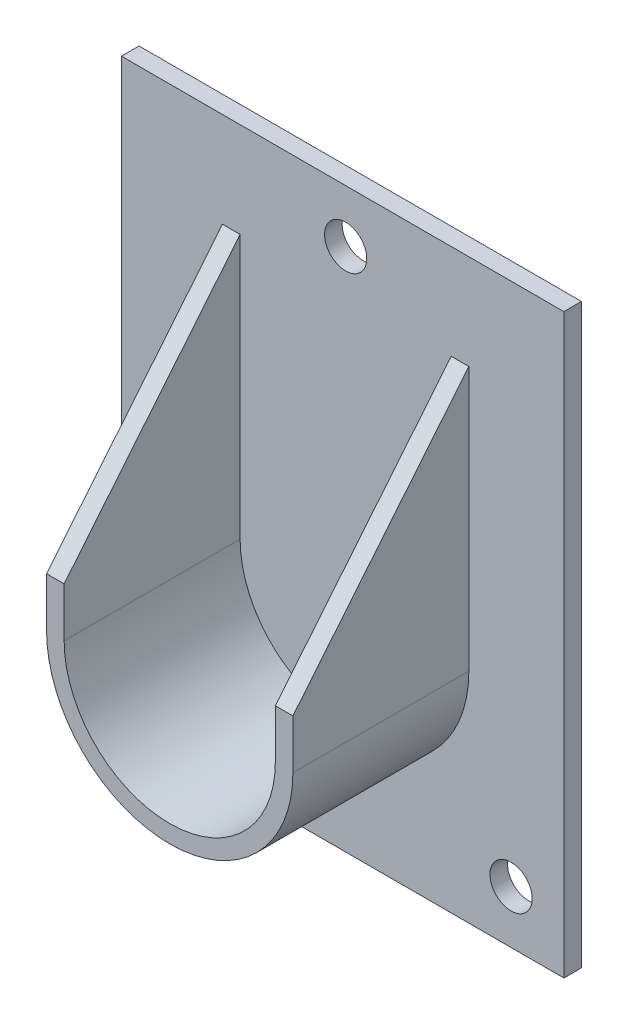
ISO-10303-21;
HEADER;
FILE_DESCRIPTION(('STEP AP214'),'2;1');
FILE_NAME('part.step','',(''),(''),'','','');
FILE_SCHEMA(('AUTOMOTIVE_DESIGN { 1 0 10303 214 1 1 1 1 }'));
ENDSEC;
DATA;
#1=APPLICATION_CONTEXT('core data for automotive mechanical design processes');
#2=APPLICATION_PROTOCOL_DEFINITION('international standard','automotive_design',2000,#1);
#3=PRODUCT_CONTEXT('',#1,'mechanical');
#4=PRODUCT('Part','Part','',(#3));
#5=PRODUCT_RELATED_PRODUCT_CATEGORY('part','',(#4));
#6=PRODUCT_DEFINITION_FORMATION('','',#4);
#7=PRODUCT_DEFINITION_CONTEXT('part definition',#1,'design');
#8=PRODUCT_DEFINITION('design','',#6,#7);
#9=PRODUCT_DEFINITION_SHAPE('','',#8);
#10=(LENGTH_UNIT() NAMED_UNIT(*) SI_UNIT(.MILLI.,.METRE.));
#11=(NAMED_UNIT(*) PLANE_ANGLE_UNIT() SI_UNIT($,.RADIAN.));
#12=(NAMED_UNIT(*) SI_UNIT($,.STERADIAN.) SOLID_ANGLE_UNIT());
#13=UNCERTAINTY_MEASURE_WITH_UNIT(LENGTH_MEASURE(1.E-05),#10,'distance_accuracy_value','');
#14=(GEOMETRIC_REPRESENTATION_CONTEXT(3) GLOBAL_UNCERTAINTY_ASSIGNED_CONTEXT((#13)) GLOBAL_UNIT_ASSIGNED_CONTEXT((#10,
#11,#12)) REPRESENTATION_CONTEXT('',''));
#15=CARTESIAN_POINT('',(0.,0.,0.));
#16=DIRECTION('',(0.,0.,1.));
#17=DIRECTION('',(1.,0.,0.));
#18=AXIS2_PLACEMENT_3D('',#15,#16,#17);
#19=CARTESIAN_POINT('',(0.,0.,55.));
#20=DIRECTION('',(0.,0.,-1.));
#21=DIRECTION('',(-1.,0.,0.));
#22=AXIS2_PLACEMENT_3D('',#19,#20,#21);
#23=CYLINDRICAL_SURFACE('',#22,30.);
#24=DIRECTION('',(0.,0.,-1.));
#25=VECTOR('',#24,1.);
#26=CARTESIAN_POINT('',(30.,0.,55.));
#27=LINE('',#26,#25);
#28=CARTESIAN_POINT('',(30.,0.,55.));
#29=VERTEX_POINT('',#28);
#30=CARTESIAN_POINT('',(30.,0.,5.));
#31=VERTEX_POINT('',#30);
#32=EDGE_CURVE('E156',#29,#31,#27,.T.);
#33=ORIENTED_EDGE('',*,*,#32,.T.);
#34=CARTESIAN_POINT('',(0.,0.,5.));
#35=DIRECTION('',(0.,0.,-1.));
#36=DIRECTION('',(-1.,0.,0.));
#37=AXIS2_PLACEMENT_3D('',#34,#35,#36);
#38=CIRCLE('',#37,30.);
#39=CARTESIAN_POINT('',(-30.,0.,5.));
#40=VERTEX_POINT('',#39);
#41=EDGE_CURVE('E52',#31,#40,#38,.T.);
#42=ORIENTED_EDGE('',*,*,#41,.T.);
#43=DIRECTION('',(0.,0.,-1.));
#44=VECTOR('',#43,1.);
#45=CARTESIAN_POINT('',(-30.,0.,55.));
#46=LINE('',#45,#44);
#47=CARTESIAN_POINT('',(-30.,0.,55.));
#48=VERTEX_POINT('',#47);
#49=EDGE_CURVE('E46',#48,#40,#46,.T.);
#50=ORIENTED_EDGE('',*,*,#49,.F.);
#51=CARTESIAN_POINT('',(0.,0.,55.));
#52=DIRECTION('',(0.,0.,1.));
#53=DIRECTION('',(1.,0.,0.));
#54=AXIS2_PLACEMENT_3D('',#51,#52,#53);
#55=CIRCLE('',#54,30.);
#56=EDGE_CURVE('E170',#48,#29,#55,.T.);
#57=ORIENTED_EDGE('',*,*,#56,.T.);
#58=EDGE_LOOP('',(#33,#42,#50,#57));
#59=FACE_BOUND('',#58,.T.);
#60=ADVANCED_FACE('F39',(#59),#23,.F.);
#61=CARTESIAN_POINT('',(-30.,0.,55.));
#62=DIRECTION('',(-1.,0.,0.));
#63=DIRECTION('',(0.,0.,1.));
#64=AXIS2_PLACEMENT_3D('',#61,#62,#63);
#65=PLANE('',#64);
#66=DIRECTION('',(0.,-1.,0.));
#67=VECTOR('',#66,1.);
#68=CARTESIAN_POINT('',(-30.,0.,5.));
#69=LINE('',#68,#67);
#70=CARTESIAN_POINT('',(-30.,75.,5.));
#71=VERTEX_POINT('',#70);
#72=EDGE_CURVE('E176',#71,#40,#69,.T.);
#73=ORIENTED_EDGE('',*,*,#72,.F.);
#74=DIRECTION('',(0.,-0.773392104960213,0.63392795488542));
#75=VECTOR('',#74,1.);
#76=CARTESIAN_POINT('',(-30.,5.62610512779296,61.8638482559074));
#77=LINE('',#76,#75);
#78=CARTESIAN_POINT('',(-30.,14.,55.));
#79=VERTEX_POINT('',#78);
#80=EDGE_CURVE('E139',#71,#79,#77,.T.);
#81=ORIENTED_EDGE('',*,*,#80,.T.);
#82=DIRECTION('',(0.,1.,0.));
#83=VECTOR('',#82,1.);
#84=CARTESIAN_POINT('',(-30.,0.,55.));
#85=LINE('',#84,#83);
#86=EDGE_CURVE('E148',#48,#79,#85,.T.);
#87=ORIENTED_EDGE('',*,*,#86,.F.);
#88=ORIENTED_EDGE('',*,*,#49,.T.);
#89=EDGE_LOOP('',(#73,#81,#87,#88));
#90=FACE_BOUND('',#89,.T.);
#91=ADVANCED_FACE('F260',(#90),#65,.F.);
#92=CARTESIAN_POINT('',(-35.,0.,55.));
#93=DIRECTION('',(-1.,0.,0.));
#94=DIRECTION('',(0.,0.,1.));
#95=AXIS2_PLACEMENT_3D('',#92,#93,#94);
#96=PLANE('',#95);
#97=DIRECTION('',(0.,-0.773392104960213,0.63392795488542));
#98=VECTOR('',#97,1.);
#99=CARTESIAN_POINT('',(-35.,5.62610512779296,61.8638482559074));
#100=LINE('',#99,#98);
#101=CARTESIAN_POINT('',(-35.,75.,5.));
#102=VERTEX_POINT('',#101);
#103=CARTESIAN_POINT('',(-35.,14.,55.));
#104=VERTEX_POINT('',#103);
#105=EDGE_CURVE('E127',#102,#104,#100,.T.);
#106=ORIENTED_EDGE('',*,*,#105,.F.);
#107=DIRECTION('',(0.,-1.,0.));
#108=VECTOR('',#107,1.);
#109=CARTESIAN_POINT('',(-35.,0.,5.));
#110=LINE('',#109,#108);
#111=CARTESIAN_POINT('',(-35.,0.,5.));
#112=VERTEX_POINT('',#111);
#113=EDGE_CURVE('E181',#102,#112,#110,.T.);
#114=ORIENTED_EDGE('',*,*,#113,.T.);
#115=DIRECTION('',(0.,0.,-1.));
#116=VECTOR('',#115,1.);
#117=CARTESIAN_POINT('',(-35.,0.,55.));
#118=LINE('',#117,#116);
#119=CARTESIAN_POINT('',(-35.,0.,55.));
#120=VERTEX_POINT('',#119);
#121=EDGE_CURVE('E155',#120,#112,#118,.T.);
#122=ORIENTED_EDGE('',*,*,#121,.F.);
#123=DIRECTION('',(0.,1.,0.));
#124=VECTOR('',#123,1.);
#125=CARTESIAN_POINT('',(-35.,0.,55.));
#126=LINE('',#125,#124);
#127=EDGE_CURVE('E145',#120,#104,#126,.T.);
#128=ORIENTED_EDGE('',*,*,#127,.T.);
#129=EDGE_LOOP('',(#106,#114,#122,#128));
#130=FACE_BOUND('',#129,.T.);
#131=ADVANCED_FACE('F147',(#130),#96,.T.);
#132=CARTESIAN_POINT('',(0.,0.,55.));
#133=DIRECTION('',(0.,0.,-1.));
#134=DIRECTION('',(-1.,0.,0.));
#135=AXIS2_PLACEMENT_3D('',#132,#133,#134);
#136=CYLINDRICAL_SURFACE('',#135,35.);
#137=CARTESIAN_POINT('',(0.,0.,5.));
#138=DIRECTION('',(0.,0.,-1.));
#139=DIRECTION('',(-1.,0.,0.));
#140=AXIS2_PLACEMENT_3D('',#137,#138,#139);
#141=CIRCLE('',#140,35.);
#142=CARTESIAN_POINT('',(35.,0.,5.));
#143=VERTEX_POINT('',#142);
#144=EDGE_CURVE('E183',#143,#112,#141,.T.);
#145=ORIENTED_EDGE('',*,*,#144,.F.);
#146=DIRECTION('',(0.,0.,-1.));
#147=VECTOR('',#146,1.);
#148=CARTESIAN_POINT('',(35.,0.,55.));
#149=LINE('',#148,#147);
#150=CARTESIAN_POINT('',(35.,0.,55.));
#151=VERTEX_POINT('',#150);
#152=EDGE_CURVE('E163',#151,#143,#149,.T.);
#153=ORIENTED_EDGE('',*,*,#152,.F.);
#154=CARTESIAN_POINT('',(0.,0.,55.));
#155=DIRECTION('',(0.,0.,1.));
#156=DIRECTION('',(1.,0.,0.));
#157=AXIS2_PLACEMENT_3D('',#154,#155,#156);
#158=CIRCLE('',#157,35.);
#159=EDGE_CURVE('E152',#120,#151,#158,.T.);
#160=ORIENTED_EDGE('',*,*,#159,.F.);
#161=ORIENTED_EDGE('',*,*,#121,.T.);
#162=EDGE_LOOP('',(#145,#153,#160,#161));
#163=FACE_BOUND('',#162,.T.);
#164=ADVANCED_FACE('F252',(#163),#136,.T.);
#165=CARTESIAN_POINT('',(35.,0.,55.));
#166=DIRECTION('',(-1.,0.,0.));
#167=DIRECTION('',(0.,0.,1.));
#168=AXIS2_PLACEMENT_3D('',#165,#166,#167);
#169=PLANE('',#168);
#170=DIRECTION('',(0.,-1.,0.));
#171=VECTOR('',#170,1.);
#172=CARTESIAN_POINT('',(35.,0.,5.));
#173=LINE('',#172,#171);
#174=CARTESIAN_POINT('',(35.,75.,5.));
#175=VERTEX_POINT('',#174);
#176=EDGE_CURVE('E187',#175,#143,#173,.T.);
#177=ORIENTED_EDGE('',*,*,#176,.F.);
#178=DIRECTION('',(0.,-0.773392104960213,0.63392795488542));
#179=VECTOR('',#178,1.);
#180=CARTESIAN_POINT('',(35.,5.62610512779296,61.8638482559074));
#181=LINE('',#180,#179);
#182=CARTESIAN_POINT('',(35.,14.,55.));
#183=VERTEX_POINT('',#182);
#184=EDGE_CURVE('E137',#175,#183,#181,.T.);
#185=ORIENTED_EDGE('',*,*,#184,.T.);
#186=DIRECTION('',(0.,1.,0.));
#187=VECTOR('',#186,1.);
#188=CARTESIAN_POINT('',(35.,0.,55.));
#189=LINE('',#188,#187);
#190=EDGE_CURVE('E158',#151,#183,#189,.T.);
#191=ORIENTED_EDGE('',*,*,#190,.F.);
#192=ORIENTED_EDGE('',*,*,#152,.T.);
#193=EDGE_LOOP('',(#177,#185,#191,#192));
#194=FACE_BOUND('',#193,.T.);
#195=ADVANCED_FACE('F247',(#194),#169,.F.);
#196=CARTESIAN_POINT('',(30.,0.,55.));
#197=DIRECTION('',(-1.,0.,0.));
#198=DIRECTION('',(0.,0.,1.));
#199=AXIS2_PLACEMENT_3D('',#196,#197,#198);
#200=PLANE('',#199);
#201=DIRECTION('',(0.,-0.773392104960213,0.63392795488542));
#202=VECTOR('',#201,1.);
#203=CARTESIAN_POINT('',(30.,5.62610512779296,61.8638482559074));
#204=LINE('',#203,#202);
#205=CARTESIAN_POINT('',(30.,75.,5.));
#206=VERTEX_POINT('',#205);
#207=CARTESIAN_POINT('',(30.,14.,55.));
#208=VERTEX_POINT('',#207);
#209=EDGE_CURVE('E150',#206,#208,#204,.T.);
#210=ORIENTED_EDGE('',*,*,#209,.F.);
#211=DIRECTION('',(0.,-1.,0.));
#212=VECTOR('',#211,1.);
#213=CARTESIAN_POINT('',(30.,0.,5.));
#214=LINE('',#213,#212);
#215=EDGE_CURVE('E11',#206,#31,#214,.T.);
#216=ORIENTED_EDGE('',*,*,#215,.T.);
#217=ORIENTED_EDGE('',*,*,#32,.F.);
#218=DIRECTION('',(0.,1.,0.));
#219=VECTOR('',#218,1.);
#220=CARTESIAN_POINT('',(30.,0.,55.));
#221=LINE('',#220,#219);
#222=EDGE_CURVE('E174',#29,#208,#221,.T.);
#223=ORIENTED_EDGE('',*,*,#222,.T.);
#224=EDGE_LOOP('',(#210,#216,#217,#223));
#225=FACE_BOUND('',#224,.T.);
#226=ADVANCED_FACE('F172',(#225),#200,.T.);
#227=CARTESIAN_POINT('',(0.,0.,55.));
#228=DIRECTION('',(0.,0.,1.));
#229=DIRECTION('',(1.,0.,0.));
#230=AXIS2_PLACEMENT_3D('',#227,#228,#229);
#231=PLANE('',#230);
#232=DIRECTION('',(1.,0.,0.));
#233=VECTOR('',#232,1.);
#234=CARTESIAN_POINT('',(-63.7172832159627,14.,55.));
#235=LINE('',#234,#233);
#236=EDGE_CURVE('E129',#104,#79,#235,.T.);
#237=ORIENTED_EDGE('',*,*,#236,.F.);
#238=ORIENTED_EDGE('',*,*,#127,.F.);
#239=ORIENTED_EDGE('',*,*,#159,.T.);
#240=ORIENTED_EDGE('',*,*,#190,.T.);
#241=EDGE_CURVE('E146',#208,#183,#235,.T.);
#242=ORIENTED_EDGE('',*,*,#241,.F.);
#243=ORIENTED_EDGE('',*,*,#222,.F.);
#244=ORIENTED_EDGE('',*,*,#56,.F.);
#245=ORIENTED_EDGE('',*,*,#86,.T.);
#246=EDGE_LOOP('',(#237,#238,#239,#240,#242,#243,#244,#245));
#247=FACE_BOUND('',#246,.T.);
#248=ADVANCED_FACE('F141',(#247),#231,.T.);
#249=CARTESIAN_POINT('',(-63.7172832159627,102.,5.));
#250=DIRECTION('',(-1.,0.,0.));
#251=DIRECTION('',(0.,-1.,0.));
#252=AXIS2_PLACEMENT_3D('',#249,#250,#251);
#253=PLANE('',#252);
#254=DIRECTION('',(0.,1.,0.));
#255=VECTOR('',#254,1.);
#256=CARTESIAN_POINT('',(-63.7172832159627,102.,0.));
#257=LINE('',#256,#255);
#258=CARTESIAN_POINT('',(-63.7172832159627,-62.,0.));
#259=VERTEX_POINT('',#258);
#260=CARTESIAN_POINT('',(-63.7172832159627,102.,0.));
#261=VERTEX_POINT('',#260);
#262=EDGE_CURVE('E209',#259,#261,#257,.T.);
#263=ORIENTED_EDGE('',*,*,#262,.F.);
#264=DIRECTION('',(0.,0.,-1.));
#265=VECTOR('',#264,1.);
#266=CARTESIAN_POINT('',(-63.7172832159627,-62.,5.));
#267=LINE('',#266,#265);
#268=CARTESIAN_POINT('',(-63.7172832159627,-62.,5.));
#269=VERTEX_POINT('',#268);
#270=EDGE_CURVE('E193',#269,#259,#267,.T.);
#271=ORIENTED_EDGE('',*,*,#270,.F.);
#272=DIRECTION('',(0.,1.,0.));
#273=VECTOR('',#272,1.);
#274=CARTESIAN_POINT('',(-63.7172832159627,102.,5.));
#275=LINE('',#274,#273);
#276=CARTESIAN_POINT('',(-63.7172832159627,102.,5.));
#277=VERTEX_POINT('',#276);
#278=EDGE_CURVE('E201',#269,#277,#275,.T.);
#279=ORIENTED_EDGE('',*,*,#278,.T.);
#280=DIRECTION('',(0.,0.,-1.));
#281=VECTOR('',#280,1.);
#282=CARTESIAN_POINT('',(-63.7172832159627,102.,5.));
#283=LINE('',#282,#281);
#284=EDGE_CURVE('E194',#277,#261,#283,.T.);
#285=ORIENTED_EDGE('',*,*,#284,.T.);
#286=EDGE_LOOP('',(#263,#271,#279,#285));
#287=FACE_BOUND('',#286,.T.);
#288=ADVANCED_FACE('F280',(#287),#253,.T.);
#289=CARTESIAN_POINT('',(62.,-62.,5.));
#290=DIRECTION('',(0.,-1.,0.));
#291=DIRECTION('',(0.,0.,-1.));
#292=AXIS2_PLACEMENT_3D('',#289,#290,#291);
#293=PLANE('',#292);
#294=DIRECTION('',(-1.,0.,0.));
#295=VECTOR('',#294,1.);
#296=CARTESIAN_POINT('',(62.,-62.,0.));
#297=LINE('',#296,#295);
#298=CARTESIAN_POINT('',(62.,-62.,0.));
#299=VERTEX_POINT('',#298);
#300=EDGE_CURVE('E199',#299,#259,#297,.T.);
#301=ORIENTED_EDGE('',*,*,#300,.F.);
#302=DIRECTION('',(0.,0.,-1.));
#303=VECTOR('',#302,1.);
#304=CARTESIAN_POINT('',(62.,-62.,5.));
#305=LINE('',#304,#303);
#306=CARTESIAN_POINT('',(62.,-62.,5.));
#307=VERTEX_POINT('',#306);
#308=EDGE_CURVE('E197',#307,#299,#305,.T.);
#309=ORIENTED_EDGE('',*,*,#308,.F.);
#310=DIRECTION('',(-1.,0.,0.));
#311=VECTOR('',#310,1.);
#312=CARTESIAN_POINT('',(62.,-62.,5.));
#313=LINE('',#312,#311);
#314=EDGE_CURVE('E191',#307,#269,#313,.T.);
#315=ORIENTED_EDGE('',*,*,#314,.T.);
#316=ORIENTED_EDGE('',*,*,#270,.T.);
#317=EDGE_LOOP('',(#301,#309,#315,#316));
#318=FACE_BOUND('',#317,.T.);
#319=ADVANCED_FACE('F281',(#318),#293,.T.);
#320=CARTESIAN_POINT('',(62.,102.,5.));
#321=DIRECTION('',(1.,0.,0.));
#322=DIRECTION('',(0.,0.,-1.));
#323=AXIS2_PLACEMENT_3D('',#320,#321,#322);
#324=PLANE('',#323);
#325=DIRECTION('',(0.,-1.,0.));
#326=VECTOR('',#325,1.);
#327=CARTESIAN_POINT('',(62.,102.,0.));
#328=LINE('',#327,#326);
#329=CARTESIAN_POINT('',(62.,102.,0.));
#330=VERTEX_POINT('',#329);
#331=EDGE_CURVE('E204',#330,#299,#328,.T.);
#332=ORIENTED_EDGE('',*,*,#331,.F.);
#333=DIRECTION('',(0.,0.,-1.));
#334=VECTOR('',#333,1.);
#335=CARTESIAN_POINT('',(62.,102.,5.));
#336=LINE('',#335,#334);
#337=CARTESIAN_POINT('',(62.,102.,5.));
#338=VERTEX_POINT('',#337);
#339=EDGE_CURVE('E195',#338,#330,#336,.T.);
#340=ORIENTED_EDGE('',*,*,#339,.F.);
#341=DIRECTION('',(0.,-1.,0.));
#342=VECTOR('',#341,1.);
#343=CARTESIAN_POINT('',(62.,102.,5.));
#344=LINE('',#343,#342);
#345=EDGE_CURVE('E216',#338,#307,#344,.T.);
#346=ORIENTED_EDGE('',*,*,#345,.T.);
#347=ORIENTED_EDGE('',*,*,#308,.T.);
#348=EDGE_LOOP('',(#332,#340,#346,#347));
#349=FACE_BOUND('',#348,.T.);
#350=ADVANCED_FACE('F287',(#349),#324,.T.);
#351=CARTESIAN_POINT('',(62.,102.,5.));
#352=DIRECTION('',(0.,1.,0.));
#353=DIRECTION('',(0.,0.,1.));
#354=AXIS2_PLACEMENT_3D('',#351,#352,#353);
#355=PLANE('',#354);
#356=DIRECTION('',(1.,0.,0.));
#357=VECTOR('',#356,1.);
#358=CARTESIAN_POINT('',(62.,102.,0.));
#359=LINE('',#358,#357);
#360=EDGE_CURVE('E210',#261,#330,#359,.T.);
#361=ORIENTED_EDGE('',*,*,#360,.F.);
#362=ORIENTED_EDGE('',*,*,#284,.F.);
#363=DIRECTION('',(1.,0.,0.));
#364=VECTOR('',#363,1.);
#365=CARTESIAN_POINT('',(62.,102.,5.));
#366=LINE('',#365,#364);
#367=EDGE_CURVE('E217',#277,#338,#366,.T.);
#368=ORIENTED_EDGE('',*,*,#367,.T.);
#369=ORIENTED_EDGE('',*,*,#339,.T.);
#370=EDGE_LOOP('',(#361,#362,#368,#369));
#371=FACE_BOUND('',#370,.T.);
#372=ADVANCED_FACE('F285',(#371),#355,.T.);
#373=CARTESIAN_POINT('',(0.,0.,5.));
#374=DIRECTION('',(0.,0.,-1.));
#375=DIRECTION('',(-1.,0.,0.));
#376=AXIS2_PLACEMENT_3D('',#373,#374,#375);
#377=PLANE('',#376);
#378=DIRECTION('',(-1.,0.,0.));
#379=VECTOR('',#378,1.);
#380=CARTESIAN_POINT('',(30.,75.,5.));
#381=LINE('',#380,#379);
#382=EDGE_CURVE('E188',#175,#206,#381,.T.);
#383=ORIENTED_EDGE('',*,*,#382,.F.);
#384=ORIENTED_EDGE('',*,*,#176,.T.);
#385=ORIENTED_EDGE('',*,*,#144,.T.);
#386=ORIENTED_EDGE('',*,*,#113,.F.);
#387=DIRECTION('',(-1.,0.,0.));
#388=VECTOR('',#387,1.);
#389=CARTESIAN_POINT('',(-35.,75.,5.));
#390=LINE('',#389,#388);
#391=EDGE_CURVE('E132',#71,#102,#390,.T.);
#392=ORIENTED_EDGE('',*,*,#391,.F.);
#393=ORIENTED_EDGE('',*,*,#72,.T.);
#394=ORIENTED_EDGE('',*,*,#41,.F.);
#395=ORIENTED_EDGE('',*,*,#215,.F.);
#396=EDGE_LOOP('',(#383,#384,#385,#386,#392,#393,#394,#395));
#397=FACE_BOUND('',#396,.T.);
#398=ORIENTED_EDGE('',*,*,#314,.F.);
#399=ORIENTED_EDGE('',*,*,#345,.F.);
#400=ORIENTED_EDGE('',*,*,#367,.F.);
#401=ORIENTED_EDGE('',*,*,#278,.F.);
#402=EDGE_LOOP('',(#398,#399,#400,#401));
#403=FACE_BOUND('',#402,.T.);
#404=CARTESIAN_POINT('',(-48.7172832159627,-47.,5.));
#405=DIRECTION('',(0.,0.,-1.));
#406=DIRECTION('',(-1.,0.,0.));
#407=AXIS2_PLACEMENT_3D('',#404,#405,#406);
#408=CIRCLE('',#407,6.);
#409=CARTESIAN_POINT('',(-54.7172832159628,-47.,5.));
#410=VERTEX_POINT('',#409);
#411=EDGE_CURVE('E213',#410,#410,#408,.T.);
#412=ORIENTED_EDGE('',*,*,#411,.T.);
#413=EDGE_LOOP('',(#412));
#414=FACE_BOUND('',#413,.T.);
#415=CARTESIAN_POINT('',(47.,-47.,5.));
#416=DIRECTION('',(0.,0.,-1.));
#417=DIRECTION('',(-1.,0.,0.));
#418=AXIS2_PLACEMENT_3D('',#415,#416,#417);
#419=CIRCLE('',#418,6.);
#420=CARTESIAN_POINT('',(41.,-47.,5.));
#421=VERTEX_POINT('',#420);
#422=EDGE_CURVE('E223',#421,#421,#419,.T.);
#423=ORIENTED_EDGE('',*,*,#422,.T.);
#424=EDGE_LOOP('',(#423));
#425=FACE_BOUND('',#424,.T.);
#426=CARTESIAN_POINT('',(0.,87.,5.));
#427=DIRECTION('',(0.,0.,-1.));
#428=DIRECTION('',(-1.,0.,0.));
#429=AXIS2_PLACEMENT_3D('',#426,#427,#428);
#430=CIRCLE('',#429,6.);
#431=CARTESIAN_POINT('',(-6.,87.,5.));
#432=VERTEX_POINT('',#431);
#433=EDGE_CURVE('E233',#432,#432,#430,.T.);
#434=ORIENTED_EDGE('',*,*,#433,.T.);
#435=EDGE_LOOP('',(#434));
#436=FACE_BOUND('',#435,.T.);
#437=ADVANCED_FACE('F251',(#397,#403,#414,#425,#436),#377,.F.);
#438=CARTESIAN_POINT('',(-48.7172832159627,-47.,5.));
#439=DIRECTION('',(0.,0.,-1.));
#440=DIRECTION('',(-1.,0.,0.));
#441=AXIS2_PLACEMENT_3D('',#438,#439,#440);
#442=CYLINDRICAL_SURFACE('',#441,6.);
#443=ORIENTED_EDGE('',*,*,#411,.F.);
#444=EDGE_LOOP('',(#443));
#445=FACE_BOUND('',#444,.T.);
#446=CARTESIAN_POINT('',(-48.7172832159627,-47.,0.));
#447=DIRECTION('',(0.,0.,-1.));
#448=DIRECTION('',(-1.,0.,0.));
#449=AXIS2_PLACEMENT_3D('',#446,#447,#448);
#450=CIRCLE('',#449,6.);
#451=CARTESIAN_POINT('',(-54.7172832159628,-47.,0.));
#452=VERTEX_POINT('',#451);
#453=EDGE_CURVE('E225',#452,#452,#450,.T.);
#454=ORIENTED_EDGE('',*,*,#453,.T.);
#455=EDGE_LOOP('',(#454));
#456=FACE_BOUND('',#455,.T.);
#457=ADVANCED_FACE('F299',(#445,#456),#442,.F.);
#458=CARTESIAN_POINT('',(47.,-47.,5.));
#459=DIRECTION('',(0.,0.,-1.));
#460=DIRECTION('',(-1.,0.,0.));
#461=AXIS2_PLACEMENT_3D('',#458,#459,#460);
#462=CYLINDRICAL_SURFACE('',#461,6.);
#463=ORIENTED_EDGE('',*,*,#422,.F.);
#464=EDGE_LOOP('',(#463));
#465=FACE_BOUND('',#464,.T.);
#466=CARTESIAN_POINT('',(47.,-47.,0.));
#467=DIRECTION('',(0.,0.,-1.));
#468=DIRECTION('',(-1.,0.,0.));
#469=AXIS2_PLACEMENT_3D('',#466,#467,#468);
#470=CIRCLE('',#469,6.);
#471=CARTESIAN_POINT('',(41.,-47.,0.));
#472=VERTEX_POINT('',#471);
#473=EDGE_CURVE('E229',#472,#472,#470,.T.);
#474=ORIENTED_EDGE('',*,*,#473,.T.);
#475=EDGE_LOOP('',(#474));
#476=FACE_BOUND('',#475,.T.);
#477=ADVANCED_FACE('F303',(#465,#476),#462,.F.);
#478=CARTESIAN_POINT('',(0.,87.,5.));
#479=DIRECTION('',(0.,0.,-1.));
#480=DIRECTION('',(-1.,0.,0.));
#481=AXIS2_PLACEMENT_3D('',#478,#479,#480);
#482=CYLINDRICAL_SURFACE('',#481,6.);
#483=ORIENTED_EDGE('',*,*,#433,.F.);
#484=EDGE_LOOP('',(#483));
#485=FACE_BOUND('',#484,.T.);
#486=CARTESIAN_POINT('',(0.,87.,0.));
#487=DIRECTION('',(0.,0.,-1.));
#488=DIRECTION('',(-1.,0.,0.));
#489=AXIS2_PLACEMENT_3D('',#486,#487,#488);
#490=CIRCLE('',#489,6.);
#491=CARTESIAN_POINT('',(-6.,87.,0.));
#492=VERTEX_POINT('',#491);
#493=EDGE_CURVE('E235',#492,#492,#490,.T.);
#494=ORIENTED_EDGE('',*,*,#493,.T.);
#495=EDGE_LOOP('',(#494));
#496=FACE_BOUND('',#495,.T.);
#497=ADVANCED_FACE('F301',(#485,#496),#482,.F.);
#498=CARTESIAN_POINT('',(0.,0.,0.));
#499=DIRECTION('',(0.,0.,1.));
#500=DIRECTION('',(1.,0.,0.));
#501=AXIS2_PLACEMENT_3D('',#498,#499,#500);
#502=PLANE('',#501);
#503=ORIENTED_EDGE('',*,*,#493,.F.);
#504=EDGE_LOOP('',(#503));
#505=FACE_BOUND('',#504,.T.);
#506=ORIENTED_EDGE('',*,*,#473,.F.);
#507=EDGE_LOOP('',(#506));
#508=FACE_BOUND('',#507,.T.);
#509=ORIENTED_EDGE('',*,*,#453,.F.);
#510=EDGE_LOOP('',(#509));
#511=FACE_BOUND('',#510,.T.);
#512=ORIENTED_EDGE('',*,*,#262,.T.);
#513=ORIENTED_EDGE('',*,*,#360,.T.);
#514=ORIENTED_EDGE('',*,*,#331,.T.);
#515=ORIENTED_EDGE('',*,*,#300,.T.);
#516=EDGE_LOOP('',(#512,#513,#514,#515));
#517=FACE_BOUND('',#516,.T.);
#518=ADVANCED_FACE('F270',(#505,#508,#511,#517),#502,.F.);
#519=CARTESIAN_POINT('',(-63.7172832159627,14.,55.));
#520=DIRECTION('',(0.,-0.63392795488542,-0.773392104960213));
#521=DIRECTION('',(0.,0.773392104960213,-0.63392795488542));
#522=AXIS2_PLACEMENT_3D('',#519,#520,#521);
#523=PLANE('',#522);
#524=ORIENTED_EDGE('',*,*,#391,.T.);
#525=ORIENTED_EDGE('',*,*,#105,.T.);
#526=ORIENTED_EDGE('',*,*,#236,.T.);
#527=ORIENTED_EDGE('',*,*,#80,.F.);
#528=EDGE_LOOP('',(#524,#525,#526,#527));
#529=FACE_BOUND('',#528,.T.);
#530=ADVANCED_FACE('F126',(#529),#523,.F.);
#531=ORIENTED_EDGE('',*,*,#382,.T.);
#532=ORIENTED_EDGE('',*,*,#209,.T.);
#533=ORIENTED_EDGE('',*,*,#241,.T.);
#534=ORIENTED_EDGE('',*,*,#184,.F.);
#535=EDGE_LOOP('',(#531,#532,#533,#534));
#536=FACE_BOUND('',#535,.T.);
#537=ADVANCED_FACE('F244',(#536),#523,.F.);
#538=CLOSED_SHELL('',(#60,#91,#131,#164,#195,#226,#248,#288,#319,#350,#372,#437,#457,#477,#497,
#518,#530,#537));
#539=MANIFOLD_SOLID_BREP('B2',#538);
#540=ADVANCED_BREP_SHAPE_REPRESENTATION('',(#18,#539),#14);
#541=SHAPE_DEFINITION_REPRESENTATION(#9,#540);
ENDSEC;
END-ISO-10303-21;
